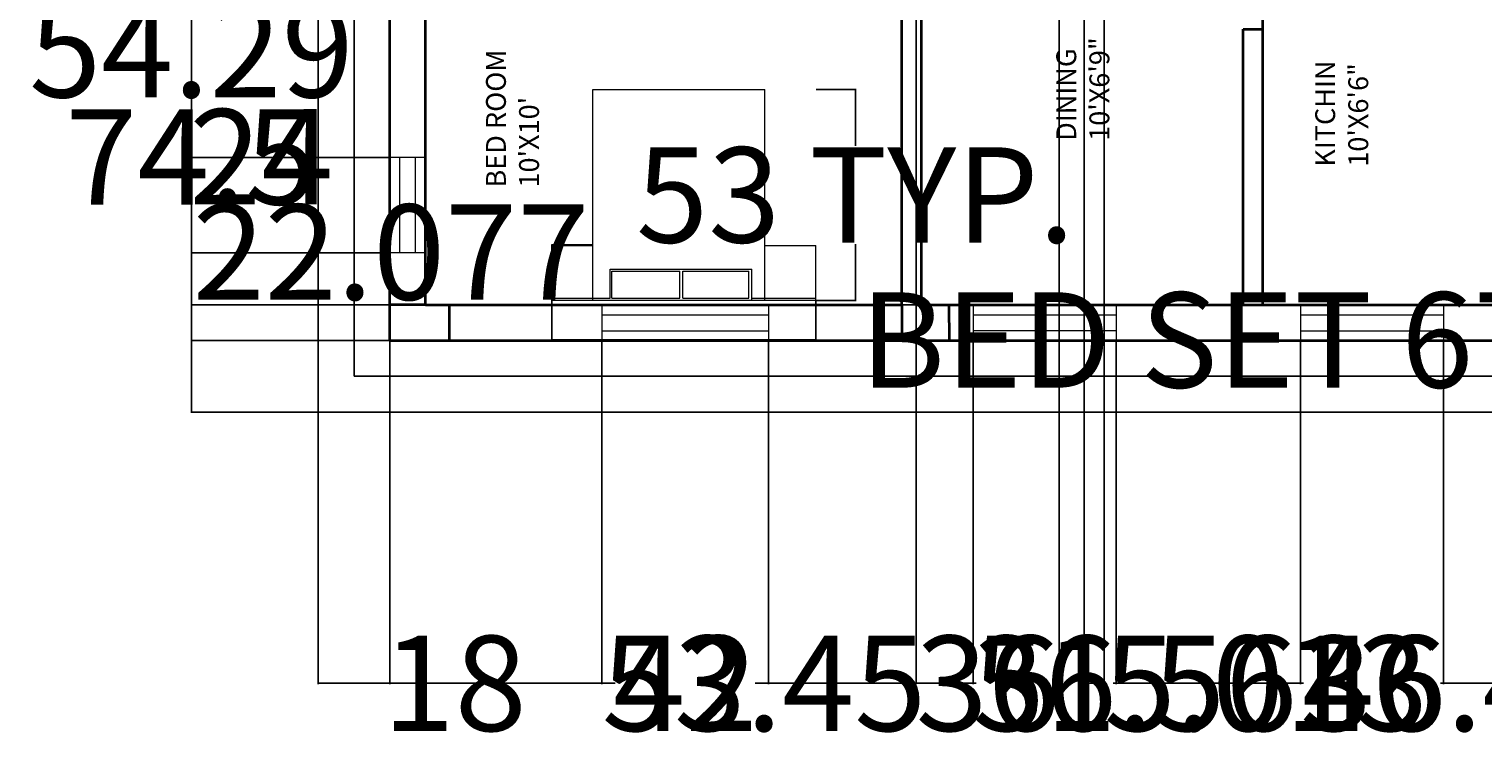
# Model space of a CAD drawing. Units: inches. Extents: x -1643 to -931, y 1907 to 2415.
# Tile 1 of 3: x -1602 to -1236, y 1907 to 2088. Entities that reach past the tile are written whole.
import ezdxf

# ---------------------------------------------------------------- set-up
doc = ezdxf.new("R2010")
doc.units = ezdxf.units.IN
for name, color, linetype, lineweight in [('A-ANNO-DIMS', 2, 'Continuous', 18), ('A-AREA-IDEN', 7, 'Continuous', 18), ('A-FURN', 8, 'Continuous', 18), ('A-GLAZ', 4, 'Continuous', 18), ('A-WALL', 7, 'Continuous', 35), ('C-PROP', 8, 'Continuous', 25)]:
    doc.layers.add(name, color=color, linetype=linetype, lineweight=lineweight)
doc.styles.get("Standard").update_dxf_attribs({"font": 'arial.ttf', "height": 24})
doc.dimstyles.get("Standard").update_dxf_attribs({"dimtxt": 0.18, "dimasz": 0.18, "dimexe": 0.18, "dimexo": 0.0625, "dimgap": 0.09, "dimtad": 0, "dimtih": 1, "dimtoh": 1, "dimdec": 4, "dimzin": 0, "dimdsep": 46, "dimtxsty": 'Standard', "dimcen": 0.09, "dimadec": 0, "dimazin": 0, "dimtfac": 1, "dimtdec": 4, "dimtofl": 0, "dimtmove": 0, "dimatfit": 3, "dimfxl": 1, "dimtolj": 1, "dimtzin": 0, "dimarcsym": 0})

# ---------------------------------------------------------------- blocks, each defined once
blk = doc.blocks.new('*U4')
for p, q in [((0, 5), (0, 0)), ((36, 5), (36, 0)), ((0, 2.5), (36, 2.5))]:
    blk.add_line(p, q)
blk = doc.blocks.new('*U8')
for p, q in [((0, 5), (0, 0)), ((42, 5), (42, 0)), ((0, 2.5), (42, 2.5))]:
    blk.add_line(p, q)
blk = doc.blocks.new('*U7')
for p, q in [((0, 5), (0, 0)), ((24, 5), (24, 0)), ((0, 2.5), (24, 2.5))]:
    blk.add_line(p, q)
blk = doc.blocks.new('BED-WITH-NIGHTSTANDS')
for p, q in [((10.33, 53.09), (53.66, 53.09)), ((10.33, 0.09), (10.33, 53.09)), ((53.66, 0.09), (53.66, 53.09)), ((0, 0), (0, 14.11)), ((0, 14.11), (10.33, 14.11)), ((0, 13.84), (10.33, 13.84)), ((53.66, 13.84), (66.5, 13.84)), ((66.5, 0.09), (66.5, 13.84)), ((14.66, 7.89), (50.39, 7.89)), ((14.66, 0.59), (14.66, 7.89)), ((15.11, 7.37), (32.28, 7.37)), ((15.11, 0.59), (15.11, 7.37)), ((32.28, 0.59), (32.28, 7.37)), ((33.01, 0.59), (33.01, 7.37)), ((33.01, 7.37), (49.65, 7.37)), ((49.65, 0.59), (49.65, 7.37)), ((50.39, 0.09), (50.39, 7.89)), ((0, 0.59), (14.66, 0.59)), ((0, 0.09), (66.5, 0.09)), ((15.11, 0.59), (32.28, 0.59)), ((33.01, 0.59), (49.65, 0.59)), ((50.39, 0.59), (66.5, 0.59))]:
    blk.add_line(p, q)
blk = doc.blocks.new('*D19')
at = {"layer": 'A-ANNO-DIMS', "color": 0, "lineweight": -2, "transparency": 16777216}
for p, q in [((-1470.32, 2019.19), (-1470.32, 2009.1)), ((-1403.82, 2019.19), (-1403.82, 2009.1)), ((-1470.14, 2009.28), (-1404, 2009.28)), ((-1403.82, 2009.28), (-1403.64, 2009.28))]:
    blk.add_line(p, q, dxfattribs=at)
at = {"layer": 'A-ANNO-DIMS', "color": 0, "transparency": 16777216}
for points in [[(-1470.14, 2009.31), (-1470.14, 2009.25), (-1470.32, 2009.28)], [(-1404, 2009.31), (-1404, 2009.25), (-1403.82, 2009.28)]]:
    blk.add_solid(points, dxfattribs=at)
at = {"layer": 'Defpoints', "color": 0, "transparency": 16777216}
for p in [(-1470.32, 2019.25), (-1403.82, 2019.25), (-1403.82, 2009.28)]:
    blk.add_point(p, dxfattribs=at)
at = {"layer": 'A-ANNO-DIMS', "color": 0, "transparency": 16777216, "insert": (-1269.29, 2009.28), "char_height": 24, "attachment_point": 5}
blk.add_mtext('\\A1;BED SET 67 TYP.', dxfattribs=at)
blk = doc.blocks.new('*D20')
at = {"layer": 'A-ANNO-DIMS', "color": 0, "lineweight": -2, "transparency": 16777216}
for p, q in [((-1403.76, 2072.34), (-1393.67, 2072.34)), ((-1393.85, 2072.16), (-1393.85, 2058.15)), ((-1393.85, 2019.43), (-1393.85, 2033.44)), ((-1403.76, 2019.25), (-1393.67, 2019.25))]:
    blk.add_line(p, q, dxfattribs=at)
at = {"layer": 'A-ANNO-DIMS', "color": 0, "transparency": 16777216}
for points in [[(-1393.88, 2072.16), (-1393.82, 2072.16), (-1393.85, 2072.34)], [(-1393.88, 2019.43), (-1393.82, 2019.43), (-1393.85, 2019.25)]]:
    blk.add_solid(points, dxfattribs=at)
at = {"layer": 'Defpoints', "color": 0, "transparency": 16777216}
for p in [(-1403.82, 2072.34), (-1393.85, 2072.34), (-1403.82, 2019.25)]:
    blk.add_point(p, dxfattribs=at)
at = {"layer": 'A-ANNO-DIMS', "color": 0, "transparency": 16777216, "insert": (-1393.85, 2045.8), "char_height": 24, "attachment_point": 5}
blk.add_mtext('\\A1;53 TYP.', dxfattribs=at)
blk = doc.blocks.new('*D22')
at = {"layer": 'A-ANNO-DIMS', "color": 0, "lineweight": -2, "transparency": 16777216}
for p, q in [((-1529.23, 2351.15), (-1561.32, 2351.15)), ((-1561.14, 2350.97), (-1561.14, 2183.5)), ((-1561.14, 1991.33), (-1561.14, 2158.79)), ((-1529.23, 1991.15), (-1561.32, 1991.15))]:
    blk.add_line(p, q, dxfattribs=at)
at = {"layer": 'A-ANNO-DIMS', "color": 0, "transparency": 16777216}
for points in [[(-1561.17, 2350.97), (-1561.11, 2350.97), (-1561.14, 2351.15)], [(-1561.17, 1991.33), (-1561.11, 1991.33), (-1561.14, 1991.15)]]:
    blk.add_solid(points, dxfattribs=at)
at = {"layer": 'Defpoints', "color": 0, "transparency": 16777216}
for p in [(-1561.14, 2351.15), (-1529.17, 2351.15), (-1529.17, 1991.15)]:
    blk.add_point(p, dxfattribs=at)
at = {"layer": 'A-ANNO-DIMS', "color": 0, "transparency": 16777216, "insert": (-1561.14, 2171.15), "char_height": 24, "attachment_point": 5}
blk.add_mtext('\\A1;360', dxfattribs=at)
blk = doc.blocks.new('*D23')
at = {"layer": 'A-ANNO-DIMS', "color": 0, "lineweight": -2, "transparency": 16777216}
for p, q in [((-1511.17, 2009.08), (-1511.17, 1922.66)), ((-1529.17, 1991.08), (-1529.17, 1922.66)), ((-1528.99, 1922.84), (-1511.35, 1922.84)), ((-1511.17, 1922.84), (-1510.99, 1922.84))]:
    blk.add_line(p, q, dxfattribs=at)
at = {"layer": 'A-ANNO-DIMS', "color": 0, "transparency": 16777216}
for points in [[(-1528.99, 1922.87), (-1528.99, 1922.81), (-1529.17, 1922.84)], [(-1511.35, 1922.87), (-1511.35, 1922.81), (-1511.17, 1922.84)]]:
    blk.add_solid(points, dxfattribs=at)
at = {"layer": 'Defpoints', "color": 0, "transparency": 16777216}
for p in [(-1511.17, 2009.15), (-1529.17, 1991.15), (-1511.17, 1922.84)]:
    blk.add_point(p, dxfattribs=at)
at = {"layer": 'A-ANNO-DIMS', "color": 0, "transparency": 16777216, "insert": (-1494.81, 1922.84), "char_height": 24, "attachment_point": 5}
blk.add_mtext('\\A1;18', dxfattribs=at)
blk = doc.blocks.new('*D35')
at = {"layer": 'A-ANNO-DIMS', "color": 0, "lineweight": -2, "transparency": 16777216}
for p, q in [((-1511.17, 2009.08), (-1511.17, 1922.66)), ((-1457.72, 2009.07), (-1457.72, 1922.66)), ((-1510.99, 1922.84), (-1457.9, 1922.84)), ((-1457.72, 1922.84), (-1457.54, 1922.84))]:
    blk.add_line(p, q, dxfattribs=at)
at = {"layer": 'A-ANNO-DIMS', "color": 0, "transparency": 16777216}
for points in [[(-1510.99, 1922.87), (-1510.99, 1922.81), (-1511.17, 1922.84)], [(-1457.9, 1922.87), (-1457.9, 1922.81), (-1457.72, 1922.84)]]:
    blk.add_solid(points, dxfattribs=at)
at = {"layer": 'Defpoints', "color": 0, "transparency": 16777216}
for p in [(-1511.17, 2009.15), (-1457.72, 2009.13), (-1457.72, 1922.84)]:
    blk.add_point(p, dxfattribs=at)
at = {"layer": 'A-ANNO-DIMS', "color": 0, "transparency": 16777216, "insert": (-1416.86, 1922.84), "char_height": 24, "attachment_point": 5}
blk.add_mtext('\\A1;53.45', dxfattribs=at)
blk = doc.blocks.new('*D36')
at = {"layer": 'A-ANNO-DIMS', "color": 0, "lineweight": -2, "transparency": 16777216}
for p, q in [((-1457.72, 2009.07), (-1457.72, 1922.66)), ((-1415.72, 2009.07), (-1415.72, 1922.66)), ((-1457.54, 1922.84), (-1454.36, 1922.84)), ((-1415.9, 1922.84), (-1419.08, 1922.84))]:
    blk.add_line(p, q, dxfattribs=at)
at = {"layer": 'A-ANNO-DIMS', "color": 0, "transparency": 16777216}
for points in [[(-1457.54, 1922.87), (-1457.54, 1922.81), (-1457.72, 1922.84)], [(-1415.9, 1922.87), (-1415.9, 1922.81), (-1415.72, 1922.84)]]:
    blk.add_solid(points, dxfattribs=at)
at = {"layer": 'Defpoints', "color": 0, "transparency": 16777216}
for p in [(-1457.72, 2009.13), (-1415.72, 2009.13), (-1415.72, 1922.84)]:
    blk.add_point(p, dxfattribs=at)
at = {"layer": 'A-ANNO-DIMS', "color": 0, "transparency": 16777216, "insert": (-1436.72, 1922.84), "char_height": 24, "attachment_point": 5}
blk.add_mtext('\\A1;42', dxfattribs=at)
blk = doc.blocks.new('*D37')
at = {"layer": 'A-ANNO-DIMS', "color": 0, "lineweight": -2, "transparency": 16777216}
for p, q in [((-1415.72, 2009.07), (-1415.72, 1922.66)), ((-1364.16, 2009.1), (-1364.16, 1922.66)), ((-1415.54, 1922.84), (-1364.34, 1922.84)), ((-1364.16, 1922.84), (-1363.98, 1922.84))]:
    blk.add_line(p, q, dxfattribs=at)
at = {"layer": 'A-ANNO-DIMS', "color": 0, "transparency": 16777216}
for points in [[(-1415.54, 1922.87), (-1415.54, 1922.81), (-1415.72, 1922.84)], [(-1364.34, 1922.87), (-1364.34, 1922.81), (-1364.16, 1922.84)]]:
    blk.add_solid(points, dxfattribs=at)
at = {"layer": 'Defpoints', "color": 0, "transparency": 16777216}
for p in [(-1415.72, 2009.13), (-1364.16, 2009.16), (-1364.16, 1922.84)]:
    blk.add_point(p, dxfattribs=at)
at = {"layer": 'A-ANNO-DIMS', "color": 0, "transparency": 16777216, "insert": (-1323.4, 1922.84), "char_height": 24, "attachment_point": 5}
blk.add_mtext('\\A1;51.56', dxfattribs=at)
blk = doc.blocks.new('*D38')
at = {"layer": 'A-ANNO-DIMS', "color": 0, "lineweight": -2, "transparency": 16777216}
for p, q in [((-1364.16, 2009.1), (-1364.16, 1922.66)), ((-1328.16, 2009.1), (-1328.16, 1922.66)), ((-1363.98, 1922.84), (-1363.42, 1922.84)), ((-1328.34, 1922.84), (-1328.9, 1922.84))]:
    blk.add_line(p, q, dxfattribs=at)
at = {"layer": 'A-ANNO-DIMS', "color": 0, "transparency": 16777216}
for points in [[(-1363.98, 1922.87), (-1363.98, 1922.81), (-1364.16, 1922.84)], [(-1328.34, 1922.87), (-1328.34, 1922.81), (-1328.16, 1922.84)]]:
    blk.add_solid(points, dxfattribs=at)
at = {"layer": 'Defpoints', "color": 0, "transparency": 16777216}
for p in [(-1364.16, 2009.16), (-1328.16, 2009.16), (-1328.16, 1922.84)]:
    blk.add_point(p, dxfattribs=at)
at = {"layer": 'A-ANNO-DIMS', "color": 0, "transparency": 16777216, "insert": (-1346.16, 1922.84), "char_height": 24, "attachment_point": 5}
blk.add_mtext('\\A1;36', dxfattribs=at)
blk = doc.blocks.new('*D39')
at = {"layer": 'A-ANNO-DIMS', "color": 0, "lineweight": -2, "transparency": 16777216}
for p, q in [((-1328.16, 2009.1), (-1328.16, 1922.66)), ((-1281.67, 2009.06), (-1281.67, 1922.66)), ((-1327.98, 1922.84), (-1281.85, 1922.84)), ((-1281.67, 1922.84), (-1281.49, 1922.84))]:
    blk.add_line(p, q, dxfattribs=at)
at = {"layer": 'A-ANNO-DIMS', "color": 0, "transparency": 16777216}
for points in [[(-1327.98, 1922.87), (-1327.98, 1922.81), (-1328.16, 1922.84)], [(-1281.85, 1922.87), (-1281.85, 1922.81), (-1281.67, 1922.84)]]:
    blk.add_solid(points, dxfattribs=at)
at = {"layer": 'Defpoints', "color": 0, "transparency": 16777216}
for p in [(-1328.16, 2009.16), (-1281.67, 2009.13), (-1281.67, 1922.84)]:
    blk.add_point(p, dxfattribs=at)
at = {"layer": 'A-ANNO-DIMS', "color": 0, "transparency": 16777216, "insert": (-1240.4, 1922.84), "char_height": 24, "attachment_point": 5}
blk.add_mtext('\\A1;46.49', dxfattribs=at)
blk = doc.blocks.new('*D40')
at = {"layer": 'A-ANNO-DIMS', "color": 0, "lineweight": -2, "transparency": 16777216}
for p, q in [((-1281.67, 2009.06), (-1281.67, 1922.66)), ((-1245.67, 2009.06), (-1245.67, 1922.66)), ((-1281.49, 1922.84), (-1280.93, 1922.84)), ((-1245.85, 1922.84), (-1246.4, 1922.84))]:
    blk.add_line(p, q, dxfattribs=at)
at = {"layer": 'A-ANNO-DIMS', "color": 0, "transparency": 16777216}
for points in [[(-1281.49, 1922.87), (-1281.49, 1922.81), (-1281.67, 1922.84)], [(-1245.85, 1922.87), (-1245.85, 1922.81), (-1245.67, 1922.84)]]:
    blk.add_solid(points, dxfattribs=at)
at = {"layer": 'Defpoints', "color": 0, "transparency": 16777216}
for p in [(-1281.67, 2009.13), (-1245.67, 2009.13), (-1245.67, 1922.84)]:
    blk.add_point(p, dxfattribs=at)
at = {"layer": 'A-ANNO-DIMS', "color": 0, "transparency": 16777216, "insert": (-1263.67, 1922.84), "char_height": 24, "attachment_point": 5}
blk.add_mtext('\\A1;36', dxfattribs=at)
blk = doc.blocks.new('*D46')
at = {"layer": 'A-ANNO-DIMS', "color": 0, "lineweight": -2, "transparency": 16777216}
for p, q in [((-1213.11, 2092.64), (-1561.32, 2092.64)), ((-1561.14, 2092.46), (-1561.14, 2067.69)), ((-1561.14, 2018.33), (-1561.14, 2043.1)), ((-1213.23, 2018.15), (-1561.32, 2018.15))]:
    blk.add_line(p, q, dxfattribs=at)
at = {"layer": 'A-ANNO-DIMS', "color": 0, "transparency": 16777216}
for points in [[(-1561.17, 2092.46), (-1561.11, 2092.46), (-1561.14, 2092.64)], [(-1561.17, 2018.33), (-1561.11, 2018.33), (-1561.14, 2018.15)]]:
    blk.add_solid(points, dxfattribs=at)
at = {"layer": 'Defpoints', "color": 0, "transparency": 16777216}
for p in [(-1213.05, 2092.64), (-1561.14, 2018.15), (-1213.17, 2018.15)]:
    blk.add_point(p, dxfattribs=at)
at = {"layer": 'A-ANNO-DIMS', "color": 0, "transparency": 16777216, "insert": (-1561.14, 2055.39), "char_height": 24, "attachment_point": 5}
blk.add_mtext('\\A1;74.5', dxfattribs=at)
blk = doc.blocks.new('*D47')
at = {"layer": 'A-ANNO-DIMS', "color": 0, "lineweight": -2, "transparency": 16777216}
for p, q in [((-1511.27, 2031.22), (-1561.32, 2031.22)), ((-1561.14, 2031.22), (-1561.14, 2031.4)), ((-1561.14, 2031.4), (-1560.96, 2031.4)), ((-1561.14, 2009.33), (-1561.14, 2031.04)), ((-1511.23, 2009.15), (-1561.32, 2009.15))]:
    blk.add_line(p, q, dxfattribs=at)
at = {"layer": 'A-ANNO-DIMS', "color": 0, "transparency": 16777216}
for points in [[(-1561.17, 2031.04), (-1561.11, 2031.04), (-1561.14, 2031.22)], [(-1561.17, 2009.33), (-1561.11, 2009.33), (-1561.14, 2009.15)]]:
    blk.add_solid(points, dxfattribs=at)
at = {"layer": 'Defpoints', "color": 0, "transparency": 16777216}
for p in [(-1561.14, 2031.22), (-1511.21, 2031.22), (-1511.17, 2009.15)]:
    blk.add_point(p, dxfattribs=at)
at = {"layer": 'A-ANNO-DIMS', "color": 0, "transparency": 16777216, "insert": (-1510.85, 2031.4), "char_height": 24, "attachment_point": 5}
blk.add_mtext('\\A1;22.077', dxfattribs=at)
blk = doc.blocks.new('*D48')
at = {"layer": 'A-ANNO-DIMS', "color": 0, "lineweight": -2, "transparency": 16777216}
for p, q in [((-1511.27, 2055.22), (-1561.32, 2055.22)), ((-1561.14, 2055.22), (-1561.14, 2055.4)), ((-1561.14, 2055.4), (-1560.96, 2055.4)), ((-1561.14, 2031.4), (-1561.14, 2055.04)), ((-1511.27, 2031.22), (-1561.32, 2031.22))]:
    blk.add_line(p, q, dxfattribs=at)
at = {"layer": 'A-ANNO-DIMS', "color": 0, "transparency": 16777216}
for points in [[(-1561.17, 2055.04), (-1561.11, 2055.04), (-1561.14, 2055.22)], [(-1561.17, 2031.4), (-1561.11, 2031.4), (-1561.14, 2031.22)]]:
    blk.add_solid(points, dxfattribs=at)
at = {"layer": 'Defpoints', "color": 0, "transparency": 16777216}
for p in [(-1561.14, 2055.22), (-1511.21, 2055.22), (-1511.21, 2031.22)]:
    blk.add_point(p, dxfattribs=at)
at = {"layer": 'A-ANNO-DIMS', "color": 0, "transparency": 16777216, "insert": (-1543.53, 2055.4), "char_height": 24, "attachment_point": 5}
blk.add_mtext('\\A1;24', dxfattribs=at)
blk = doc.blocks.new('*D49')
at = {"layer": 'A-ANNO-DIMS', "color": 0, "lineweight": -2, "transparency": 16777216}
for p, q in [((-1511.21, 2109.52), (-1561.32, 2109.52)), ((-1561.14, 2109.34), (-1561.14, 2094.71)), ((-1561.14, 2055.4), (-1561.14, 2070.03)), ((-1511.27, 2055.22), (-1561.32, 2055.22))]:
    blk.add_line(p, q, dxfattribs=at)
at = {"layer": 'A-ANNO-DIMS', "color": 0, "transparency": 16777216}
for points in [[(-1561.17, 2109.34), (-1561.11, 2109.34), (-1561.14, 2109.52)], [(-1561.17, 2055.4), (-1561.11, 2055.4), (-1561.14, 2055.22)]]:
    blk.add_solid(points, dxfattribs=at)
at = {"layer": 'Defpoints', "color": 0, "transparency": 16777216}
for p in [(-1561.14, 2109.52), (-1511.15, 2109.52), (-1511.21, 2055.22)]:
    blk.add_point(p, dxfattribs=at)
at = {"layer": 'A-ANNO-DIMS', "color": 0, "transparency": 16777216, "insert": (-1561.14, 2082.37), "char_height": 24, "attachment_point": 5}
blk.add_mtext('\\A1;54.29', dxfattribs=at)
blk = doc.blocks.new('*D55')
at = {"layer": 'A-ANNO-DIMS', "color": 0, "lineweight": -2, "transparency": 16777216}
for p, q in [((-1378.5, 2191.08), (-1378.5, 1922.66)), ((-1342.5, 2191.08), (-1342.5, 1922.66)), ((-1378.32, 1922.84), (-1377.76, 1922.84)), ((-1342.68, 1922.84), (-1343.23, 1922.84))]:
    blk.add_line(p, q, dxfattribs=at)
at = {"layer": 'A-ANNO-DIMS', "color": 0, "transparency": 16777216}
for points in [[(-1378.32, 1922.87), (-1378.32, 1922.81), (-1378.5, 1922.84)], [(-1342.68, 1922.87), (-1342.68, 1922.81), (-1342.5, 1922.84)]]:
    blk.add_solid(points, dxfattribs=at)
at = {"layer": 'Defpoints', "color": 0, "transparency": 16777216}
for p in [(-1378.5, 2191.15), (-1342.5, 2191.15), (-1342.5, 1922.84)]:
    blk.add_point(p, dxfattribs=at)
at = {"layer": 'A-ANNO-DIMS', "color": 0, "transparency": 16777216, "insert": (-1360.5, 1922.84), "char_height": 24, "attachment_point": 5}
blk.add_mtext('\\A1;36', dxfattribs=at)
blk = doc.blocks.new('*D62')
at = {"layer": 'A-ANNO-DIMS', "color": 0, "lineweight": -2, "transparency": 16777216}
for p, q in [((-1336.17, 2196.08), (-1336.17, 1922.66)), ((-1331.15, 2191.08), (-1331.15, 1922.66)), ((-1335.99, 1922.84), (-1331.33, 1922.84)), ((-1331.15, 1922.84), (-1330.97, 1922.84))]:
    blk.add_line(p, q, dxfattribs=at)
at = {"layer": 'A-ANNO-DIMS', "color": 0, "transparency": 16777216}
for points in [[(-1335.99, 1922.87), (-1335.99, 1922.81), (-1336.17, 1922.84)], [(-1331.33, 1922.87), (-1331.33, 1922.81), (-1331.15, 1922.84)]]:
    blk.add_solid(points, dxfattribs=at)
at = {"layer": 'Defpoints', "color": 0, "transparency": 16777216}
for p in [(-1336.17, 2196.15), (-1331.15, 2191.15), (-1331.15, 1922.84)]:
    blk.add_point(p, dxfattribs=at)
at = {"layer": 'A-ANNO-DIMS', "color": 0, "transparency": 16777216, "insert": (-1290.39, 1922.84), "char_height": 24, "attachment_point": 5}
blk.add_mtext('\\A1;5.013', dxfattribs=at)
blk = doc.blocks.new('*D63')
at = {"layer": 'A-ANNO-DIMS', "color": 0, "lineweight": -2, "transparency": 16777216}
for p, q in [((-1245.67, 2009.06), (-1245.67, 1922.66)), ((-1208.17, 2009.08), (-1208.17, 1922.66)), ((-1245.49, 1922.84), (-1208.35, 1922.84)), ((-1208.17, 1922.84), (-1207.99, 1922.84))]:
    blk.add_line(p, q, dxfattribs=at)
at = {"layer": 'A-ANNO-DIMS', "color": 0, "transparency": 16777216}
for points in [[(-1245.49, 1922.87), (-1245.49, 1922.81), (-1245.67, 1922.84)], [(-1208.35, 1922.87), (-1208.35, 1922.81), (-1208.17, 1922.84)]]:
    blk.add_solid(points, dxfattribs=at)
at = {"layer": 'Defpoints', "color": 0, "transparency": 16777216}
for p in [(-1245.67, 2009.13), (-1208.17, 2009.15), (-1208.17, 1922.84)]:
    blk.add_point(p, dxfattribs=at)
at = {"layer": 'A-ANNO-DIMS', "color": 0, "transparency": 16777216, "insert": (-1176.64, 1922.84), "char_height": 24, "attachment_point": 5}
blk.add_mtext('\\A1;37.5', dxfattribs=at)

msp = doc.modelspace()

# ---------------------------------------------------------------- linework, layer by layer
at = {"layer": 'A-WALL'}
for p, q in [((-1511.1668, 2009.1464), (-1511.1668, 2306.1464)), ((-1502.1668, 2018.1464), (-1502.1668, 2138.1464)), ((-1382.1668, 2018.1464), (-1382.1668, 2138.1464)), ((-1377.1668, 2018.1464), (-1377.1668, 2138.1464)), ((-1291.1668, 2018.1464), (-1291.1668, 2138.1464)), ((-1296.1668, 2018.1464), (-1296.1668, 2087.5551)), ((-1296.1668, 2087.5551), (-1291.1668, 2087.5551)), ((-1496.1628, 2018.2716), (-1496.1628, 2008.9001)), ((-1370.3225, 2018.2765), (-1370.2247, 2008.9859)), ((-1502.1668, 2018.1464), (-1511.1668, 2018.1464)), ((-1502.1668, 2018.1464), (-1382.1668, 2018.1464)), ((-1382.1668, 2018.1464), (-1382.1668, 2009.1464)), ((-1377.1668, 2018.1464), (-1136.1668, 2018.1464)), ((-1511.1668, 2009.1464), (-1131.1668, 2009.1464))]:
    msp.add_line(p, q, dxfattribs=at)
at = {"layer": 'C-PROP'}
for p, q in [((-1529.1668, 1991.1464), (-1529.1668, 2351.1464)), ((-1520.1668, 2000.1464), (-1520.1668, 2342.1464)), ((-1520.1668, 2000.1464), (-1058.1668, 2000.1464)), ((-1529.1668, 1991.1464), (-1049.1668, 1991.1464))]:
    msp.add_line(p, q, dxfattribs=at)

# ---------------------------------------------------------------- block references
at = {"layer": 'A-FURN'}
msp.add_blockref('BED-WITH-NIGHTSTANDS', (-1470.325, 2019.252), dxfattribs=at)
at = {"layer": 'A-GLAZ', "rotation": 270}
for p in [(-1511.2115, 2055.2238), (-1507.2375, 2055.239)]:
    msp.add_blockref('*U7', p, dxfattribs=at)
at = {"layer": 'A-GLAZ'}
for name, p in [('*U8', (-1457.7194, 2013.143)), ('*U4', (-1364.1588, 2013.0948)), ('*U4', (-1281.6758, 2013.0948)), ('*U8', (-1457.7173, 2009.1293)), ('*U4', (-1364.1588, 2009.1602)), ('*U4', (-1281.6674, 2009.1256))]:
    msp.add_blockref(name, p, dxfattribs=at)

# ---------------------------------------------------------------- texts
at = {"layer": 'A-AREA-IDEN', "char_height": 5, "attachment_point": 1, "rotation": 90}
for s, width, insert in [('DINING\\P10\'X6\'9"', 50.968553, (-1343.2135, 2059.4223)), ("BED ROOM\\P10'X10'", 153.656396, (-1486.9061, 2047.665)), ('KITCHIN\\P10\'X6\'6"', 93.616064, (-1277.9861, 2052.9105))]:
    msp.add_mtext_dynamic_manual_height_columns(s, width=width, gutter_width=120, heights=[0], dxfattribs=dict(at, insert=insert))

# ---------------------------------------------------------------- dimensions: what is measured, and where the dimension line sits
at = {"layer": 'A-ANNO-DIMS'}
for base, p1, p2, override, picture, middle in [((-1561.1409, 2351.1464), (-1529.1668, 1991.1464), (-1529.1668, 2351.1464), {"dimdec": 0, "dimlfac": 1, "dimrnd": 0, "dimzin": 0, "dimdsep": 46, "dimlunit": 2}, '*D22', (-1561.1409, 2171.1464)), ((-1561.1409, 2109.516), (-1511.2115, 2055.2238), (-1511.1453, 2109.516), {"dimdec": 2, "dimlfac": 1, "dimrnd": 0, "dimzin": 0, "dimdsep": 46, "dimlunit": 2}, '*D49', (-1561.1409, 2082.3699)), ((-1561.1409, 2018.1464), (-1213.047, 2092.64), (-1213.1668, 2018.1464), {"dimdec": 1, "dimlfac": 1, "dimrnd": 0, "dimzin": 0, "dimdsep": 46, "dimlunit": 2}, '*D46', (-1561.1409, 2055.3932)), ((-1561.1409, 2055.2238), (-1511.2115, 2031.2238), (-1511.2115, 2055.2238), {"dimdec": 0, "dimlfac": 1, "dimrnd": 0, "dimzin": 0, "dimdsep": 46, "dimlunit": 2}, '*D48', (-1543.5258, 2055.4038)), ((-1561.1409, 2031.2238), (-1511.1668, 2009.1464), (-1511.2115, 2031.2238), {"dimdec": 3, "dimlfac": 1, "dimrnd": 0, "dimzin": 0, "dimdsep": 46, "dimlunit": 2}, '*D47', (-1510.8491, 2031.4038))]:
    dim = msp.add_linear_dim(base=base, p1=p1, p2=p2, angle=90, dimstyle='Standard', override=override, dxfattribs=at)
    dim.commit()
    dim.dimension.update_dxf_attribs({"geometry": picture, "text_midpoint": middle})
for base, p1, p2, override, picture, middle in [((-1331.1542, 1922.8359), (-1336.1668, 2196.1464), (-1331.1542, 2191.1464), {"dimdec": 3, "dimlfac": 1, "dimrnd": 0, "dimzin": 0, "dimdsep": 46, "dimlunit": 2}, '*D62', (-1290.3903, 1922.8359)), ((-1342.4982, 1922.8359), (-1378.4982, 2191.1464), (-1342.4982, 2191.1464), {"dimdec": 0, "dimlfac": 1, "dimrnd": 0, "dimzin": 0, "dimdsep": 46, "dimlunit": 2}, '*D55', (-1360.4982, 1922.8359)), ((-1511.1668, 1922.8359), (-1529.1668, 1991.1464), (-1511.1668, 2009.1464), {"dimdec": 0, "dimlfac": 1, "dimrnd": 0, "dimzin": 0, "dimdsep": 46, "dimlunit": 2}, '*D23', (-1494.8123, 1922.8359)), ((-1457.7173, 1922.8359), (-1511.1668, 2009.1464), (-1457.7173, 2009.1293), {"dimdec": 2, "dimlfac": 1, "dimrnd": 0, "dimzin": 0, "dimdsep": 46, "dimlunit": 2}, '*D35', (-1416.8634, 1922.8359)), ((-1415.7173, 1922.8359), (-1457.7173, 2009.1293), (-1415.7173, 2009.1293), {"dimdec": 0, "dimlfac": 1, "dimrnd": 0, "dimzin": 0, "dimdsep": 46, "dimlunit": 2}, '*D36', (-1436.7173, 1922.8359)), ((-1364.1588, 1922.8359), (-1415.7173, 2009.1293), (-1364.1588, 2009.1602), {"dimdec": 2, "dimlfac": 1, "dimrnd": 0, "dimzin": 0, "dimdsep": 46, "dimlunit": 2}, '*D37', (-1323.4032, 1922.8359)), ((-1328.1588, 1922.8359), (-1364.1588, 2009.1602), (-1328.1588, 2009.1602), {"dimdec": 0, "dimlfac": 1, "dimrnd": 0, "dimzin": 0, "dimdsep": 46, "dimlunit": 2}, '*D38', (-1346.1588, 1922.8359)), ((-1281.6674, 1922.8359), (-1328.1588, 2009.1602), (-1281.6674, 2009.1256), {"dimdec": 2, "dimlfac": 1, "dimrnd": 0, "dimzin": 0, "dimdsep": 46, "dimlunit": 2}, '*D39', (-1240.396, 1922.8359)), ((-1245.6674, 1922.8359), (-1281.6674, 2009.1256), (-1245.6674, 2009.1256), {"dimdec": 0, "dimlfac": 1, "dimrnd": 0, "dimzin": 0, "dimdsep": 46, "dimlunit": 2}, '*D40', (-1263.6674, 1922.8359)), ((-1208.1668, 1922.8359), (-1245.6674, 2009.1256), (-1208.1668, 2009.1464), {"dimdec": 1, "dimlfac": 1, "dimrnd": 0, "dimzin": 0, "dimdsep": 46, "dimlunit": 2}, '*D63', (-1176.6445, 1922.8359))]:
    dim = msp.add_linear_dim(base=base, p1=p1, p2=p2, dimstyle='Standard', override=override, dxfattribs=at)
    dim.commit()
    dim.dimension.update_dxf_attribs({"geometry": picture, "text_midpoint": middle})
dim = msp.add_linear_dim(base=(-1403.8243, 2009.277), p1=(-1470.3248, 2019.2521), p2=(-1403.8243, 2019.2521), text='BED SET <> TYP.', dimstyle='Standard', override={"dimdec": 0, "dimlfac": 1, "dimrnd": 0, "dimzin": 0, "dimdsep": 46, "dimlunit": 2}, dxfattribs=at)
dim.commit()
dim.dimension.update_dxf_attribs({"geometry": '*D19', "text_midpoint": (-1269.2869, 2009.277)})
dim = msp.add_linear_dim(base=(-1393.8492, 2072.3407), p1=(-1403.8243, 2019.2521), p2=(-1403.8243, 2072.3407), angle=90, text='<> TYP.', dimstyle='Standard', override={"dimdec": 0, "dimlfac": 1, "dimrnd": 0, "dimzin": 0, "dimdsep": 46, "dimlunit": 2}, dxfattribs=at)
dim.commit()
dim.dimension.update_dxf_attribs({"geometry": '*D20', "text_midpoint": (-1393.8492, 2045.7964)})

doc.saveas('drawing.dxf')
